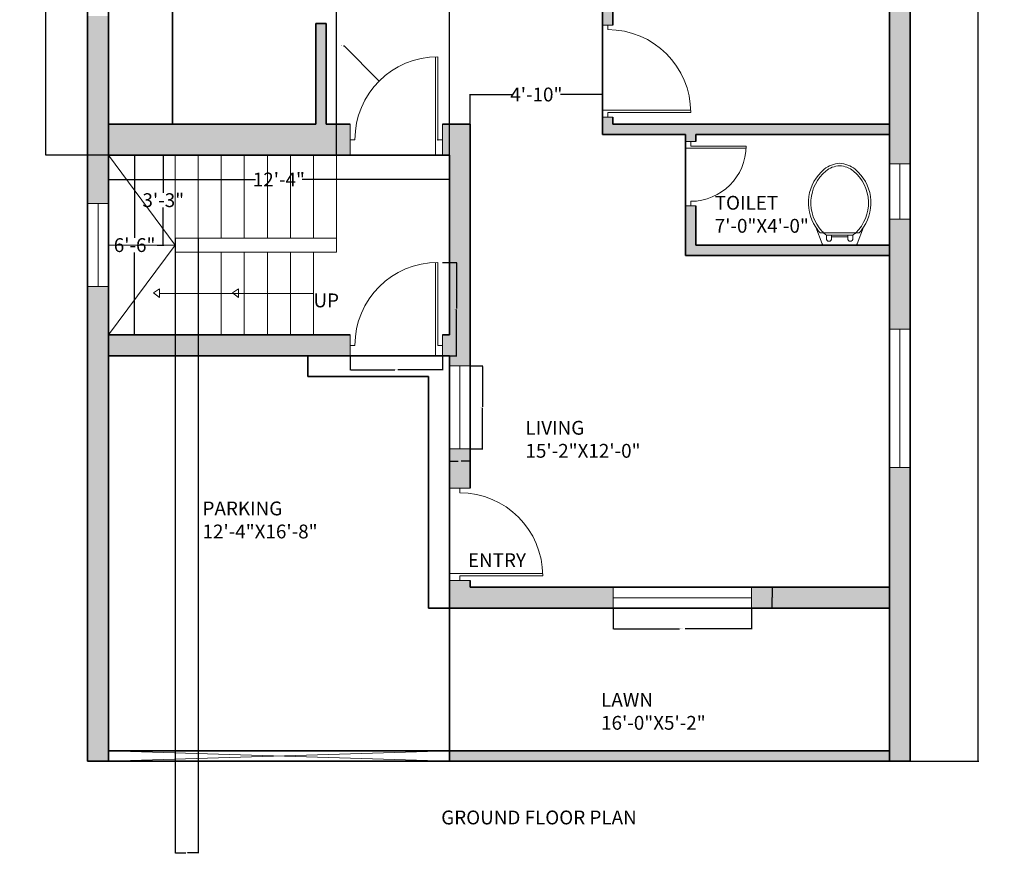
# Model space of a CAD drawing. Units: inches. Extents: x -15 to 423, y -713 to 71.
# Tile 1 of 24: x -4 to 423, y -713 to -351. Entities that reach past the tile are written whole.
import ezdxf

# ---------------------------------------------------------------- set-up
doc = ezdxf.new("R2010")
doc.units = ezdxf.units.IN
doc.header["$MEASUREMENT"] = 0
for name, color, linetype, lineweight in [('A-ANNO-DIMS', 2, 'Continuous', 18), ('A-ANNO-SYMB', 7, 'Continuous', 13), ('A-ANNO-TEXT', 7, 'Continuous', 18), ('A-AREA-IDEN', 7, 'Continuous', 18), ('A-DOOR', 3, 'Continuous', 18), ('A-FLOR-CASE', 7, 'Continuous', 25), ('A-FLOR-STRS', 7, 'Continuous', 18), ('A-GLAZ', 5, 'Continuous', 18), ('A-SITE-GATE', 1, 'Continuous', 18), ('A-WALL', 7, 'Continuous', 35), ('A-WALL-PATT', 8, 'Continuous', 13), ('WC-Detail_dwgmodels.com', 251, 'Continuous', 13), ('WC-Outline_dwgmodels.com', 250, 'Continuous', 18)]:
    doc.layers.add(name, color=color, linetype=linetype, lineweight=lineweight)
doc.styles.get("Standard").update_dxf_attribs({"font": 'arial.ttf'})
doc.dimstyles.get("Standard").update_dxf_attribs({"dimtxt": 0.18, "dimasz": 0.18, "dimexe": 0.18, "dimexo": 0.0625, "dimgap": 0.09, "dimtad": 0, "dimtih": 1, "dimtoh": 1, "dimdec": 0, "dimzin": 0, "dimdsep": 46, "dimlunit": 3, "dimtxsty": 'Standard', "dimcen": 0.09, "dimadec": 0, "dimazin": 0, "dimtfac": 1, "dimtdec": 0, "dimtofl": 0, "dimtmove": 0, "dimatfit": 3, "dimfxl": 1, "dimtolj": 1, "dimtzin": 0, "dimarcsym": 0})

# ---------------------------------------------------------------- blocks, each defined once
blk = doc.blocks.new('*D3')
at = {"layer": 'A-ANNO-DIMS', "color": 0, "lineweight": -2, "transparency": 16777216}
for p, q in [((34.08, -413.18), (34.08, -420.72)), ((182.08, -413.18), (182.08, -420.72)), ((34.26, -420.54), (97.97, -420.54)), ((181.9, -420.54), (118.19, -420.54))]:
    blk.add_line(p, q, dxfattribs=at)
at = {"layer": 'A-ANNO-DIMS', "color": 0, "transparency": 16777216}
for points in [[(34.26, -420.51), (34.26, -420.57), (34.08, -420.54)], [(181.9, -420.51), (181.9, -420.57), (182.08, -420.54)]]:
    blk.add_solid(points, dxfattribs=at)
at = {"layer": 'Defpoints', "color": 0, "transparency": 16777216}
for p in [(34.08, -413.12), (182.08, -413.12), (182.08, -420.54)]:
    blk.add_point(p, dxfattribs=at)
at = {"layer": 'A-ANNO-DIMS', "color": 0, "transparency": 16777216, "insert": (108.08, -420.54), "char_height": 6, "attachment_point": 5}
blk.add_mtext('\\A1;12\'-4"', dxfattribs=at)
blk = doc.blocks.new('*D4')
at = {"layer": 'A-ANNO-DIMS', "color": 0, "lineweight": -2, "transparency": 16777216}
for p, q in [((50.57, -410), (45.28, -410)), ((45.46, -410.18), (45.46, -445.85)), ((45.46, -487.82), (45.46, -452.15)), ((50.57, -488), (45.28, -488))]:
    blk.add_line(p, q, dxfattribs=at)
at = {"layer": 'A-ANNO-DIMS', "color": 0, "transparency": 16777216}
for points in [[(45.43, -410.18), (45.49, -410.18), (45.46, -410)], [(45.43, -487.82), (45.49, -487.82), (45.46, -488)]]:
    blk.add_solid(points, dxfattribs=at)
at = {"layer": 'Defpoints', "color": 0, "transparency": 16777216}
for p in [(50.63, -410), (45.46, -488), (50.63, -488)]:
    blk.add_point(p, dxfattribs=at)
at = {"layer": 'A-ANNO-DIMS', "color": 0, "transparency": 16777216, "insert": (45.46, -449), "char_height": 6, "attachment_point": 5}
blk.add_mtext('\\A1;6\'-6"', dxfattribs=at)
blk = doc.blocks.new('*D5')
at = {"layer": 'A-ANNO-DIMS', "color": 0, "lineweight": -2, "transparency": 16777216}
for p, q in [((55.24, -410), (58.09, -410)), ((57.91, -410.18), (57.91, -426.34)), ((57.91, -448.82), (57.91, -432.66)), ((55.24, -449), (58.09, -449))]:
    blk.add_line(p, q, dxfattribs=at)
at = {"layer": 'A-ANNO-DIMS', "color": 0, "transparency": 16777216}
for points in [[(57.88, -410.18), (57.94, -410.18), (57.91, -410)], [(57.88, -448.82), (57.94, -448.82), (57.91, -449)]]:
    blk.add_solid(points, dxfattribs=at)
at = {"layer": 'Defpoints', "color": 0, "transparency": 16777216}
for p in [(55.18, -410), (55.18, -449), (57.91, -449)]:
    blk.add_point(p, dxfattribs=at)
at = {"layer": 'A-ANNO-DIMS', "color": 0, "transparency": 16777216, "insert": (57.91, -429.5), "char_height": 6, "attachment_point": 5}
blk.add_mtext('\\A1;3\'-3"', dxfattribs=at)
blk = doc.blocks.new('*D6')
at = {"layer": 'A-ANNO-DIMS', "color": 0, "lineweight": -2, "transparency": 16777216}
for p, q in [((191.08, -396.44), (191.08, -383.46)), ((191.26, -383.64), (209.31, -383.64)), ((248.4, -383.64), (230.35, -383.64)), ((248.58, -393.44), (248.58, -383.46))]:
    blk.add_line(p, q, dxfattribs=at)
at = {"layer": 'A-ANNO-DIMS', "color": 0, "transparency": 16777216}
for points in [[(191.26, -383.61), (191.26, -383.67), (191.08, -383.64)], [(248.4, -383.61), (248.4, -383.67), (248.58, -383.64)]]:
    blk.add_solid(points, dxfattribs=at)
at = {"layer": 'Defpoints', "color": 0, "transparency": 16777216}
for p in [(248.58, -383.64), (191.08, -396.5), (248.58, -393.5)]:
    blk.add_point(p, dxfattribs=at)
at = {"layer": 'A-ANNO-DIMS', "color": 0, "transparency": 16777216, "insert": (219.83, -383.64), "char_height": 6, "attachment_point": 5}
blk.add_mtext('\\A1;4\'-10"', dxfattribs=at)
blk = doc.blocks.new('*D8')
at = {"layer": 'A-ANNO-DIMS', "color": 0, "lineweight": -2, "transparency": 16777216}
for p, q in [((25.02, 17.5), (6.72, 17.5)), ((6.9, 17.32), (6.9, -193.09)), ((6.9, -409.82), (6.9, -199.41)), ((34.02, -410), (6.72, -410))]:
    blk.add_line(p, q, dxfattribs=at)
at = {"layer": 'A-ANNO-DIMS', "color": 0, "transparency": 16777216}
for points in [[(6.87, 17.32), (6.93, 17.32), (6.9, 17.5)], [(6.87, -409.82), (6.93, -409.82), (6.9, -410)]]:
    blk.add_solid(points, dxfattribs=at)
at = {"layer": 'Defpoints', "color": 0, "transparency": 16777216}
for p in [(25.08, 17.5), (6.9, -410), (34.08, -410)]:
    blk.add_point(p, dxfattribs=at)
at = {"layer": 'A-ANNO-DIMS', "color": 0, "transparency": 16777216, "insert": (6.9, -196.25), "char_height": 6, "attachment_point": 5}
blk.add_mtext('\\A1;35\'-8"', dxfattribs=at)
blk = doc.blocks.new('*D9')
at = {"layer": 'A-ANNO-DIMS', "color": 0, "lineweight": -2, "transparency": 16777216}
for p, q in [((382.14, 17.5), (411.79, 17.5)), ((411.61, 17.32), (411.61, -324.61)), ((411.61, -672.82), (411.61, -330.89)), ((382.14, -673), (411.79, -673))]:
    blk.add_line(p, q, dxfattribs=at)
at = {"layer": 'A-ANNO-DIMS', "color": 0, "transparency": 16777216}
for points in [[(411.58, 17.32), (411.64, 17.32), (411.61, 17.5)], [(411.58, -672.82), (411.64, -672.82), (411.61, -673)]]:
    blk.add_solid(points, dxfattribs=at)
at = {"layer": 'Defpoints', "color": 0, "transparency": 16777216}
for p in [(382.08, 17.5), (382.08, -673), (411.61, -673)]:
    blk.add_point(p, dxfattribs=at)
at = {"layer": 'A-ANNO-DIMS', "color": 0, "transparency": 16777216, "insert": (411.61, -327.75), "char_height": 6, "attachment_point": 5}
blk.add_mtext('\\A1;57\'-7"', dxfattribs=at)
blk = doc.blocks.new('WINDOW-60IN')
for p, q in [((0, 9), (60, 9)), ((0, 0), (0, 9)), ((60, 9), (60, 0)), ((0, 4.5), (60, 4.5)), ((60, 0), (0, 0))]:
    blk.add_line(p, q)
blk = doc.blocks.new('WINDOW-24IN')
for p, q in [((9, 24), (0, 24)), ((0, 24), (0, 0)), ((4.5, 0), (4.5, 24)), ((9, 0), (9, 24)), ((0, 0), (9, 0))]:
    blk.add_line(p, q)
blk = doc.blocks.new('WINDOW-36IN')
for p, q in [((0, 36), (0, 0)), ((9, 36), (0, 36)), ((4.5, 36), (4.5, 0)), ((9, 0), (9, 36)), ((0, 0), (9, 0))]:
    blk.add_line(p, q)
blk = doc.blocks.new('DOOR-24IN-JAMB4_5')
for p, q in [((25, 0), (25, 26.25)), ((26, 2.25), (26, 26.25)), ((0, 2.25), (0, 4.5)), ((28, 4.5), (28, 0)), ((2, 2.25), (0, 2.25)), ((0, 2.25), (0, 0)), ((28, 2.25), (26, 2.25))]:
    blk.add_line(p, q)
blk.add_arc((26, 2.25), 24, 90, 180)
blk = doc.blocks.new('DOOR-36IN-JAMB4_5')
for p, q in [((2, 2.25), (2, 38.25)), ((3, 0), (3, 38.25)), ((0, 4.5), (0, 0)), ((40, 2.25), (40, 4.5)), ((0, 2.25), (2, 2.25)), ((38, 2.25), (40, 2.25)), ((40, 2.25), (40, 0))]:
    blk.add_line(p, q)
blk.add_arc((2, 2.25), 36, 0, 90)
blk = doc.blocks.new('DOOR-36IN-JAMB9')
for p, q in [((37, 0), (37, 40.5)), ((38, 4.5), (38, 40.5)), ((0, 4.5), (0, 9)), ((40, 9), (40, 0)), ((2, 4.5), (0, 4.5)), ((0, 4.5), (0, 0)), ((40, 4.5), (38, 4.5))]:
    blk.add_line(p, q)
blk.add_arc((38, 4.5), 36, 90, 180)
blk = doc.blocks.new('STAIR-DIRECTION-ARROW')
for p, q in [((2.56, 3.79), (0, 2.02)), ((0, 2.02), (2.56, 0)), ((2.56, 1.7), (2.56, 3.79)), ((2.56, 0), (2.56, 1.7))]:
    blk.add_line(p, q)
blk = doc.blocks.new('*D19')
at = {"layer": 'A-ANNO-DIMS', "color": 0, "lineweight": -2, "transparency": 16777216}
for p, q in [((253.2, -606.56), (253.2, -615.68)), ((313.2, -606.56), (313.2, -615.68)), ((253.38, -615.5), (281.97, -615.5)), ((313.02, -615.5), (284.43, -615.5))]:
    blk.add_line(p, q, dxfattribs=at)
at = {"layer": 'A-ANNO-DIMS', "color": 0, "transparency": 16777216}
for points in [[(253.38, -615.47), (253.38, -615.53), (253.2, -615.5)], [(313.02, -615.47), (313.02, -615.53), (313.2, -615.5)]]:
    blk.add_solid(points, dxfattribs=at)
at = {"layer": 'Defpoints', "color": 0, "transparency": 16777216}
for p in [(253.2, -606.5), (313.2, -606.5), (313.2, -615.5)]:
    blk.add_point(p, dxfattribs=at)
at = {"layer": 'A-ANNO-DIMS', "color": 0, "transparency": 16777216, "insert": (283.2, -615.5), "char_height": 0.18, "attachment_point": 5}
blk.add_mtext('\\A1;WINDOW 5\'-0" TYP.', dxfattribs=at)
blk = doc.blocks.new('*D20')
at = {"layer": 'A-ANNO-DIMS', "color": 0, "lineweight": -2, "transparency": 16777216}
for p, q in [((313.26, -597.5), (322.38, -597.5)), ((322.2, -597.68), (322.2, -601.82)), ((322.2, -606.32), (322.2, -602.18)), ((313.26, -606.5), (322.38, -606.5))]:
    blk.add_line(p, q, dxfattribs=at)
at = {"layer": 'A-ANNO-DIMS', "color": 0, "transparency": 16777216}
for points in [[(322.17, -597.68), (322.23, -597.68), (322.2, -597.5)], [(322.17, -606.32), (322.23, -606.32), (322.2, -606.5)]]:
    blk.add_solid(points, dxfattribs=at)
at = {"layer": 'Defpoints', "color": 0, "transparency": 16777216}
for p in [(313.2, -597.5), (322.2, -597.5), (313.2, -606.5)]:
    blk.add_point(p, dxfattribs=at)
at = {"layer": 'A-ANNO-DIMS', "color": 0, "transparency": 16777216, "insert": (322.2, -602), "char_height": 0.18, "attachment_point": 5}
blk.add_mtext('\\A1;0\'-9" TYP.', dxfattribs=at)
blk = doc.blocks.new('*D21')
at = {"layer": 'A-ANNO-DIMS', "color": 0, "lineweight": -2, "transparency": 16777216}
for p, q in [((191.14, -501.43), (196.66, -501.43)), ((196.48, -501.61), (196.48, -519.25)), ((196.48, -537.25), (196.48, -519.61)), ((191.14, -537.43), (196.66, -537.43))]:
    blk.add_line(p, q, dxfattribs=at)
at = {"layer": 'A-ANNO-DIMS', "color": 0, "transparency": 16777216}
for points in [[(196.45, -501.61), (196.51, -501.61), (196.48, -501.43)], [(196.45, -537.25), (196.51, -537.25), (196.48, -537.43)]]:
    blk.add_solid(points, dxfattribs=at)
at = {"layer": 'Defpoints', "color": 0, "transparency": 16777216}
for p in [(191.08, -501.43), (196.48, -501.43), (191.08, -537.43)]:
    blk.add_point(p, dxfattribs=at)
at = {"layer": 'A-ANNO-DIMS', "color": 0, "transparency": 16777216, "insert": (196.48, -519.43), "char_height": 0.18, "attachment_point": 5}
blk.add_mtext('\\A1;WINDOW 3\'-0" TYP.', dxfattribs=at)
blk = doc.blocks.new('*D22')
at = {"layer": 'A-ANNO-DIMS', "color": 0, "lineweight": -2, "transparency": 16777216}
for p, q in [((182.08, -537.49), (182.08, -543.01)), ((191.08, -537.49), (191.08, -543.01)), ((182.26, -542.83), (185.94, -542.83)), ((190.9, -542.83), (187.22, -542.83))]:
    blk.add_line(p, q, dxfattribs=at)
at = {"layer": 'A-ANNO-DIMS', "color": 0, "transparency": 16777216}
for points in [[(182.26, -542.8), (182.26, -542.86), (182.08, -542.83)], [(190.9, -542.8), (190.9, -542.86), (191.08, -542.83)]]:
    blk.add_solid(points, dxfattribs=at)
at = {"layer": 'Defpoints', "color": 0, "transparency": 16777216}
for p in [(182.08, -537.43), (191.08, -537.43), (191.08, -542.83)]:
    blk.add_point(p, dxfattribs=at)
at = {"layer": 'A-ANNO-DIMS', "color": 0, "transparency": 16777216, "insert": (186.58, -542.83), "char_height": 0.18, "attachment_point": 5}
blk.add_mtext('\\A1;0\'-9" TYP.', dxfattribs=at)
blk = doc.blocks.new('*D29')
at = {"layer": 'A-ANNO-DIMS', "color": 0, "lineweight": -2, "transparency": 16777216}
for p, q in [((179.14, -456.5), (185.34, -456.5)), ((185.16, -456.68), (185.16, -476.57)), ((185.16, -496.82), (185.16, -476.93)), ((179.14, -497), (185.34, -497))]:
    blk.add_line(p, q, dxfattribs=at)
at = {"layer": 'A-ANNO-DIMS', "color": 0, "transparency": 16777216}
for points in [[(185.13, -456.68), (185.19, -456.68), (185.16, -456.5)], [(185.13, -496.82), (185.19, -496.82), (185.16, -497)]]:
    blk.add_solid(points, dxfattribs=at)
at = {"layer": 'Defpoints', "color": 0, "transparency": 16777216}
for p in [(179.08, -456.5), (185.16, -456.5), (179.08, -497)]:
    blk.add_point(p, dxfattribs=at)
at = {"layer": 'A-ANNO-DIMS', "color": 0, "transparency": 16777216, "insert": (185.16, -476.75), "char_height": 0.18, "attachment_point": 5}
blk.add_mtext('\\A1;DOOR 3\'-4 1/2" TYP.', dxfattribs=at)
blk = doc.blocks.new('*D30')
at = {"layer": 'A-ANNO-DIMS', "color": 0, "lineweight": -2, "transparency": 16777216}
for p, q in [((139.08, -497.06), (139.08, -503.25)), ((179.08, -497.06), (179.08, -503.25)), ((139.26, -503.07), (158.44, -503.07)), ((178.9, -503.07), (159.72, -503.07))]:
    blk.add_line(p, q, dxfattribs=at)
at = {"layer": 'A-ANNO-DIMS', "color": 0, "transparency": 16777216}
for points in [[(139.26, -503.04), (139.26, -503.1), (139.08, -503.07)], [(178.9, -503.04), (178.9, -503.1), (179.08, -503.07)]]:
    blk.add_solid(points, dxfattribs=at)
at = {"layer": 'Defpoints', "color": 0, "transparency": 16777216}
for p in [(139.08, -497), (179.08, -497), (179.08, -503.07)]:
    blk.add_point(p, dxfattribs=at)
at = {"layer": 'A-ANNO-DIMS', "color": 0, "transparency": 16777216, "insert": (159.08, -503.07), "char_height": 0.18, "attachment_point": 5}
blk.add_mtext('\\A1;3\'-4" TYP.', dxfattribs=at)
blk = doc.blocks.new('*D37')
at = {"layer": 'A-ANNO-DIMS', "color": 0, "lineweight": -2, "transparency": 16777216}
for p, q in [((34.08, -396.44), (34.08, 57.43)), ((34.26, 57.25), (47.65, 57.25)), ((61.7, 57.25), (48.31, 57.25)), ((61.88, -396.44), (61.88, 57.43))]:
    blk.add_line(p, q, dxfattribs=at)
at = {"layer": 'A-ANNO-DIMS', "color": 0, "transparency": 16777216}
for points in [[(34.26, 57.28), (34.26, 57.22), (34.08, 57.25)], [(61.7, 57.28), (61.7, 57.22), (61.88, 57.25)]]:
    blk.add_solid(points, dxfattribs=at)
at = {"layer": 'Defpoints', "color": 0, "transparency": 16777216}
for p in [(61.88, 57.25), (34.08, -396.5), (61.88, -396.5)]:
    blk.add_point(p, dxfattribs=at)
at = {"layer": 'A-ANNO-DIMS', "color": 0, "transparency": 16777216, "insert": (47.98, 57.25), "char_height": 0.18, "attachment_point": 5}
blk.add_mtext('\\A1;2\'-4"', dxfattribs=at)
blk = doc.blocks.new('*D41')
at = {"layer": 'A-ANNO-DIMS', "color": 0, "lineweight": -2, "transparency": 16777216}
for p, q in [((63.08, -446.06), (63.08, -712.93)), ((73.08, -446.06), (73.08, -712.93)), ((63.26, -712.75), (67.68, -712.75)), ((72.9, -712.75), (68.48, -712.75))]:
    blk.add_line(p, q, dxfattribs=at)
at = {"layer": 'A-ANNO-DIMS', "color": 0, "transparency": 16777216}
for points in [[(63.26, -712.72), (63.26, -712.78), (63.08, -712.75)], [(72.9, -712.72), (72.9, -712.78), (73.08, -712.75)]]:
    blk.add_solid(points, dxfattribs=at)
at = {"layer": 'Defpoints', "color": 0, "transparency": 16777216}
for p in [(63.08, -446), (73.08, -446), (73.08, -712.75)]:
    blk.add_point(p, dxfattribs=at)
at = {"layer": 'A-ANNO-DIMS', "color": 0, "transparency": 16777216, "insert": (68.08, -712.75), "char_height": 0.18, "attachment_point": 5}
blk.add_mtext('\\A1;0\'-10"', dxfattribs=at)
blk = doc.blocks.new('*D42')
at = {"layer": 'A-ANNO-DIMS', "color": 0, "lineweight": -2, "transparency": 16777216}
for p, q in [((133.08, -409.94), (133.08, 57.43)), ((133.26, 57.25), (157.25, 57.25)), ((181.9, 57.25), (157.91, 57.25)), ((182.08, -409.94), (182.08, 57.43))]:
    blk.add_line(p, q, dxfattribs=at)
at = {"layer": 'A-ANNO-DIMS', "color": 0, "transparency": 16777216}
for points in [[(133.26, 57.28), (133.26, 57.22), (133.08, 57.25)], [(181.9, 57.28), (181.9, 57.22), (182.08, 57.25)]]:
    blk.add_solid(points, dxfattribs=at)
at = {"layer": 'Defpoints', "color": 0, "transparency": 16777216}
for p in [(182.08, 57.25), (133.08, -410), (182.08, -410)]:
    blk.add_point(p, dxfattribs=at)
at = {"layer": 'A-ANNO-DIMS', "color": 0, "transparency": 16777216, "insert": (157.58, 57.25), "char_height": 0.18, "attachment_point": 5}
blk.add_mtext('\\A1;4\'-1"', dxfattribs=at)
blk = doc.blocks.new('*D43')
at = {"layer": 'A-ANNO-DIMS', "color": 0, "lineweight": -2, "transparency": 16777216}
for p, q in [((136.17, -362.52), (136.35, -362.52)), ((136.35, -362.52), (151.5, -377.67)), ((176.99, -403.25), (177.17, -403.25)), ((177.08, -403.34), (177.08, -403.16))]:
    blk.add_line(p, q, dxfattribs=at)
at = {"layer": 'A-ANNO-DIMS', "color": 0, "transparency": 16777216}
blk.add_solid([(151.52, -377.65), (151.48, -377.69), (151.62, -377.79)], dxfattribs=at)
at = {"layer": 'Defpoints', "color": 0, "transparency": 16777216}
for p in [(151.62, -377.79), (177.08, -403.25)]:
    blk.add_point(p, dxfattribs=at)
at = {"layer": 'A-ANNO-DIMS', "color": 0, "transparency": 16777216, "insert": (135.56, -362.52), "char_height": 0.18, "attachment_point": 5}
blk.add_mtext('\\A1;3X R3\'-0"', dxfattribs=at)

msp = doc.modelspace()

# ---------------------------------------------------------------- hatches: boundary and pattern name
at = {"layer": 'A-WALL-PATT'}
h = msp.add_hatch(color=256, dxfattribs=at)
h.dxf.hatch_style = 1
h.paths.add_polyline_path([(34.08, -349.58), (25.08, -349.58), (25.08, -431), (34.08, -431)])
h.paths.add_polyline_path([(34.08, -467), (25.08, -467), (25.08, -673), (34.08, -673)])
h.paths.add_polyline_path([(373.08, -668.5), (182.08, -668.5), (182.08, -673), (373.08, -673)])
h.paths.add_polyline_path([(253.2, -597.5), (191.08, -597.5), (191.08, -594.5), (182.08, -594.5), (182.08, -606.5), (253.2, -606.5)])
h.paths.add_polyline_path([(373.08, -597.5), (313.2, -597.5), (313.2, -606.5), (373.08, -606.5)])
h.paths.add_polyline_path([(382.08, -545.55), (373.08, -545.55), (373.08, -673), (382.08, -673)])
h.paths.add_polyline_path([(139.08, -488), (34.08, -488), (34.08, -497), (139.08, -497), (139.08, -492.5)])
h.paths.add_polyline_path([(139.08, -396.5), (128.58, -396.5), (128.58, -352.79), (124.08, -352.79), (124.08, -396.5), (34.08, -396.5), (34.08, -410), (139.08, -410), (139.08, -403.25)])
h.paths.add_polyline_path([(191.08, -396.5), (179.08, -396.5), (179.08, -410), (182.08, -410), (182.08, -488), (179.08, -488), (179.08, -497), (182.08, -497), (182.08, -501.43), (191.08, -501.43)])
h.paths.add_polyline_path([(373.08, -396.5), (253.08, -396.5), (253.08, -393.5), (248.58, -393.5), (248.58, -401), (284.58, -401), (284.58, -404), (289.08, -404), (289.08, -401), (373.08, -401)])
h.paths.add_polyline_path([(373.08, -449), (289.08, -449), (289.08, -432), (286.83, -432), (284.58, -432), (284.58, -453.5), (373.08, -453.5)])
h.paths.add_polyline_path([(382.08, -344.27), (373.08, -344.27), (373.08, -413.68), (382.08, -413.68)])
h.paths.add_polyline_path([(382.08, -437.68), (373.08, -437.68), (373.08, -485.55), (382.08, -485.55)])
h.paths.add_polyline_path([(34.08, -188.26), (25.08, -188.26), (25.08, -289.58), (34.08, -289.58)])
h.paths.add_polyline_path([(164.08, -236), (34.08, -236), (34.08, -240.5), (124.08, -240.5), (124.08, -293.12), (128.58, -293.12), (128.58, -240.5), (164.08, -240.5), (164.08, -238.25)])
h.paths.add_polyline_path([(373.08, -236), (242.58, -236), (242.58, -238.25), (242.58, -240.5), (248.58, -240.5), (248.58, -353.5), (250.83, -353.5), (253.08, -353.5), (253.08, -240.5), (373.08, -240.5)])
h.paths.add_polyline_path([(382.08, -190.86), (373.08, -190.86), (373.08, -284.27), (382.08, -284.27)])
h.paths.add_polyline_path([(211.58, -80), (253.58, -80), (253.58, -77.75), (253.58, -75.5), (153.58, -75.5), (153.58, -77.75), (153.58, -80), (207.08, -80), (207.08, -236), (204.08, -236), (204.08, -240.5), (214.58, -240.5), (214.58, -236), (211.58, -236)])
h.paths.add_polyline_path([(34.08, 8.5), (70.36, 8.5), (70.36, 17.5), (25.08, 17.5), (25.08, -128.26), (34.08, -128.26)])
h.paths.add_polyline_path([(110.58, 17.5), (94.36, 17.5), (94.36, 8.5), (110.58, 8.5)])
h.paths.add_polyline_path([(296.58, 17.5), (110.58, 17.5), (110.58, 13), (296.58, 13)])
h.paths.add_polyline_path([(110.58, 8.5), (106.08, 8.5), (106.08, -75.5), (103.08, -75.5), (103.08, -80), (113.58, -80), (113.58, -77.75), (113.58, -75.5), (110.58, -75.5)])
h.paths.add_polyline_path([(75.08, -75.5), (34.08, -75.5), (34.08, -80), (75.08, -80), (75.08, -77.75)])
h.paths.add_polyline_path([(343.09, 17.5), (296.58, 17.5), (296.58, 13), (296.58, 8.5), (343.09, 8.5)])
h.paths.add_polyline_path([(304.08, -75.5), (301.08, -75.5), (301.08, 8.5), (296.58, 8.5), (296.58, -75.5), (293.58, -75.5), (293.58, -80), (304.08, -80)])
h.paths.add_polyline_path([(382.08, 17.5), (367.09, 17.5), (367.09, 8.5), (373.08, 8.5), (373.08, -130.86), (382.08, -130.86)])
h.paths.add_polyline_path([(373.08, -75.5), (332.08, -75.5), (332.08, -77.75), (332.08, -80), (373.08, -80)])
h = msp.add_hatch(color=256, dxfattribs=at)
h.dxf.hatch_style = 1
h.paths.add_polyline_path([(191.08, -537.43), (182.08, -537.43), (182.08, -554.5), (186.58, -554.5), (191.08, -554.5)])

# ---------------------------------------------------------------- linework, layer by layer
at = {"layer": 'A-ANNO-SYMB'}
msp.add_line((123.08, -470), (56.22, -470), dxfattribs=at)
at = {"layer": 'A-DOOR'}
for p, q in [((176.08, -410), (176.08, -367.25)), ((177.08, -403.25), (177.08, -367.25)), ((139.08, -403.25), (139.08, -396.5)), ((179.08, -410), (179.08, -396.5)), ((141.08, -403.25), (139.08, -403.25)), ((139.08, -403.25), (139.08, -410)), ((179.08, -403.25), (177.08, -403.25))]:
    msp.add_line(p, q, dxfattribs=at)
msp.add_arc((177.08, -403.25), 36, 90, 180, dxfattribs=at)
at = {"layer": 'A-FLOR-CASE'}
msp.add_line((61.88, -275.98), (61.88, -396.5), dxfattribs=at)
at = {"layer": 'A-FLOR-STRS'}
for p, q in [((63.08, -449), (34.08, -410)), ((63.08, -410), (63.08, -488)), ((73.08, -410), (73.08, -446)), ((83.08, -410), (83.08, -446)), ((93.08, -410), (93.08, -446)), ((103.08, -410), (103.08, -446)), ((113.08, -410), (113.08, -446)), ((123.08, -410), (123.08, -446)), ((133.08, -410), (133.08, -452)), ((63.08, -446), (133.08, -446)), ((63.08, -449), (34.08, -449)), ((63.08, -449), (34.08, -488)), ((63.08, -452), (133.08, -452)), ((73.08, -452), (73.08, -488)), ((83.08, -452), (83.08, -488)), ((93.08, -452), (93.08, -488)), ((103.08, -452), (103.08, -488)), ((113.08, -452), (113.08, -488)), ((123.08, -452), (123.08, -488))]:
    msp.add_line(p, q, dxfattribs=at)
at = {"layer": 'A-SITE-GATE'}
for p, q in [((34.08, -668.5), (182.08, -673)), ((182.08, -668.5), (34.08, -673))]:
    msp.add_line(p, q, dxfattribs=at)
at = {"layer": 'A-WALL'}
for p, q in [((25.08, 17.5), (25.08, -673)), ((382.08, 17.5), (382.08, -673)), ((34.08, 8.5), (34.08, -673)), ((373.08, 8.5), (373.08, -673)), ((248.58, -240.5), (248.58, -401)), ((253.08, -240.5), (253.08, -353.5)), ((124.08, -352.79), (128.58, -352.79)), ((124.08, -352.79), (124.08, -396.5)), ((128.58, -352.79), (128.58, -396.5)), ((34.08, -396.5), (124.08, -396.5)), ((128.58, -396.5), (139.08, -396.5)), ((179.08, -396.5), (191.08, -396.5)), ((191.08, -396.5), (191.08, -554.5)), ((253.08, -393.5), (253.08, -396.5)), ((253.08, -396.5), (373.08, -396.5)), ((248.58, -401), (284.58, -401)), ((284.58, -401), (284.58, -453.5)), ((289.08, -401), (373.08, -401)), ((289.08, -401), (289.08, -404)), ((34.08, -410), (182.08, -410)), ((182.08, -410), (182.08, -488)), ((289.08, -432), (289.08, -449)), ((289.08, -449), (373.08, -449)), ((284.58, -453.5), (373.08, -453.5)), ((34.08, -488), (139.08, -488)), ((179.08, -488), (182.08, -488)), ((34.08, -497), (182.08, -497)), ((120.64, -497), (120.64, -506)), ((182.08, -497), (182.08, -668.5)), ((120.64, -506), (173.08, -506)), ((173.08, -506), (173.08, -606.5)), ((191.08, -594.5), (191.08, -597.5)), ((191.08, -597.5), (373.08, -597.5)), ((173.08, -606.5), (182.08, -606.5)), ((182.08, -606.5), (373.08, -606.5)), ((34.08, -668.5), (373.08, -668.5)), ((182.08, -668.5), (182.08, -673)), ((25.08, -673), (382.08, -673))]:
    msp.add_line(p, q, dxfattribs=at)
at = {"layer": 'WC-Detail_dwgmodels.com'}
for p, q in [((342.98, -443.63), (344.47, -443.63)), ((358.44, -443.63), (359.93, -443.63))]:
    msp.add_line(p, q, dxfattribs=at)
for points in [[(342.98, -443.63, -0.040937), (341.06, -441.19, -0.163732)], [(345.7, -444.7, -0.022712), (344.47, -443.63, -0.162618)], [(357.21, -444.7, 0.022712), (358.44, -443.63, 0.162618)], [(359.93, -443.63, 0.040937), (361.85, -441.19, 0.163732)], [(351.45, -444.7), (345.7, -444.7, -0.022712)], [(345.7, -444.7), (345.7, -446.19, 1), (347.96, -446.19), (347.96, -445.41)], [(351.45, -444.7), (357.21, -444.7, 0.476108)], [(357.21, -444.7), (357.21, -446.19, -1), (354.95, -446.19), (354.95, -445.41)]]:
    msp.add_lwpolyline(points, format="xyb", dxfattribs=at)
for points in [[(347.96, -445.41), (347.96, -444.7)], [(354.95, -445.41), (347.96, -445.41)], [(354.95, -445.41), (354.95, -444.7)]]:
    msp.add_lwpolyline(points, dxfattribs=at)
at = {"layer": 'WC-Outline_dwgmodels.com'}
for p in [(344.47, -443.63), (358.44, -443.63)]:
    msp.add_line(p, (351.45, -443.63), dxfattribs=at)
for points in [[(341.06, -441.19, -0.383919), (344.78, -416.07, -0.163732), (351.45, -413.51, -0.359733)], [(361.85, -441.19, 0.383919), (358.13, -416.07, 0.163732), (351.45, -413.51, 0.359733)], [(343.76, -442.9, -0.431639), (345.46, -416.88, -0.162618), (351.45, -414.57, -0.470877)], [(358.44, -443.63, 0.448546), (357.45, -416.88, 0.162618), (351.45, -414.57, 0.470877)], [(351.45, -449), (344.68, -449, -0.31031), (343.85, -448.43), (341.06, -441.19, -0.209071)], [(344.47, -443.63, -0.014165), (343.76, -442.9, -0.162618)], [(351.45, -449), (358.23, -449, 0.31031), (359.06, -448.43), (361.85, -441.19, 0.209071)]]:
    msp.add_lwpolyline(points, format="xyb", dxfattribs=at)

# ---------------------------------------------------------------- block references
at = {"layer": 'A-ANNO-SYMB'}
for p in [(53.66, -471.7), (88.01, -471.7)]:
    msp.add_blockref('STAIR-DIRECTION-ARROW', p, dxfattribs=at)
at = {"layer": 'A-DOOR', "extrusion": (0, 0, -1), "zscale": -1, "rotation": 90.00000000000003}
for name, p in [('DOOR-36IN-JAMB4_5', (-248.58, -393.5)), ('DOOR-24IN-JAMB4_5', (-284.58, -432))]:
    msp.add_blockref(name, p, dxfattribs=at)
at = {"layer": 'A-DOOR'}
msp.add_blockref('DOOR-36IN-JAMB9', (139.08, -497), dxfattribs=at)
at = {"layer": 'A-DOOR', "rotation": 270}
msp.add_blockref('DOOR-36IN-JAMB9', (182.08, -554.5), dxfattribs=at)
at = {"layer": 'A-GLAZ'}
for name, p in [('WINDOW-24IN', (373.08, -437.68)), ('WINDOW-36IN', (25.08, -467)), ('WINDOW-36IN', (182.08, -537.43)), ('WINDOW-60IN', (253.2, -606.5))]:
    msp.add_blockref(name, p, dxfattribs=at)
at = {"layer": 'A-GLAZ', "rotation": 90.00000000000011}
msp.add_blockref('WINDOW-60IN', (382.08, -545.55), dxfattribs=at)

# ---------------------------------------------------------------- texts
at = {"layer": 'A-ANNO-TEXT', "char_height": 6, "attachment_point": 1}
for s, insert in [('UP', (123.08, -470)), ('GROUND FLOOR PLAN', (178.53, -694.38))]:
    msp.add_mtext(s, dxfattribs=dict(at, insert=insert))
at = {"layer": 'A-AREA-IDEN', "char_height": 6, "attachment_point": 1}
for s, insert in [('TOILET\\P7\'-0"X4\'-0"', (297.24, -427.63)), ('LIVING\\P15\'-2"X12\'-0"', (215.1, -525.27)), ('PARKING\\P12\'-4"X16\'-8"', (74.94, -560.28)), ('ENTRY', (190.13, -582.75)), ('LAWN\\P16\'-0"X5\'-2"', (247.92, -643.31))]:
    msp.add_mtext(s, dxfattribs=dict(at, insert=insert))

# ---------------------------------------------------------------- dimensions: what is measured, and where the dimension line sits
at = {"layer": 'A-ANNO-DIMS'}
for base, p1, p2, override, picture, middle in [((61.88, 57.25), (34.08, -396.5), (61.88, -396.5), {"dimdec": 1, "dimlfac": 1, "dimrnd": 0, "dimzin": 1, "dimdsep": 46, "dimlunit": 4, "dimfrac": 2}, '*D37', (47.98, 57.25)), ((182.08, 57.25), (133.08, -410), (182.08, -410), {"dimdec": 1, "dimlfac": 1, "dimrnd": 0, "dimzin": 1, "dimdsep": 46, "dimlunit": 4, "dimfrac": 2}, '*D42', (157.58, 57.25)), ((248.58055573, -383.64367342), (191.08055573, -396.49989936), (248.58055573, -393.49989936), {"dimtxt": 6, "dimclrd": 0, "dimclre": 0, "dimclrt": 0}, '*D6', (219.83055573, -383.64367342)), ((182.08, -420.54), (34.08, -413.12), (182.08, -413.12), {"dimtxt": 6, "dimclrd": 0, "dimclre": 0, "dimclrt": 0}, '*D3', (108.08, -420.54)), ((73.08, -712.75), (63.08, -446), (73.08, -446), {"dimdec": 1, "dimlfac": 1, "dimrnd": 0, "dimzin": 1, "dimdsep": 46, "dimlunit": 4, "dimfrac": 2}, '*D41', (68.08, -712.75))]:
    dim = msp.add_linear_dim(base=base, p1=p1, p2=p2, dimstyle='Standard', override=override, dxfattribs=at)
    dim.commit()
    dim.dimension.update_dxf_attribs({"geometry": picture, "text_midpoint": middle})
for base, p1, p2, picture, middle in [((6.9041327, -409.99989936), (25.08055573, 17.50010064), (34.08055573, -409.99989936), '*D8', (6.9041327, -196.24989936)), ((411.6050599, -672.99989936), (382.08055573, 17.50010064), (382.08055573, -672.99989936), '*D9', (411.6050599, -327.74989936)), ((45.46, -488), (50.63, -410), (50.63, -488), '*D4', (45.46, -449)), ((57.91, -449), (55.18, -410), (55.18, -449), '*D5', (57.91, -429.5))]:
    dim = msp.add_linear_dim(base=base, p1=p1, p2=p2, angle=90, dimstyle='Standard', override={"dimtxt": 6, "dimclrd": 0, "dimclre": 0, "dimclrt": 0}, dxfattribs=at)
    dim.commit()
    dim.dimension.update_dxf_attribs({"geometry": picture, "text_midpoint": middle})
dim = msp.add_radius_dim(center=(177.08, -403.25), mpoint=(151.62, -377.79), text='3X <>', dimstyle='Standard', override={"dimdec": 1, "dimlfac": 1, "dimrnd": 0, "dimzin": 1, "dimdsep": 46, "dimlunit": 4, "dimfrac": 2}, dxfattribs=at)
dim.commit()
dim.dimension.update_dxf_attribs({"geometry": '*D43', "text_midpoint": (135.56, -362.52), "dimtype": 164})
for base, p1, p2, text, picture, middle in [((185.16, -456.5), (179.08, -497), (179.08, -456.5), 'DOOR <> TYP.', '*D29', (185.16, -476.75)), ((196.48, -501.43), (191.08, -537.43), (191.08, -501.43), 'WINDOW <> TYP.', '*D21', (196.48, -519.43)), ((322.2, -597.5), (313.2, -606.5), (313.2, -597.5), '<> TYP.', '*D20', (322.2, -602))]:
    dim = msp.add_linear_dim(base=base, p1=p1, p2=p2, angle=90, text=text, dimstyle='Standard', override={"dimdec": 1, "dimlfac": 1, "dimrnd": 0, "dimzin": 1, "dimdsep": 46, "dimlunit": 4, "dimfrac": 2}, dxfattribs=at)
    dim.commit()
    dim.dimension.update_dxf_attribs({"geometry": picture, "text_midpoint": middle})
for base, p1, p2, text, picture, middle in [((179.08, -503.07), (139.08, -497), (179.08, -497), '<> TYP.', '*D30', (159.08, -503.07)), ((191.08, -542.83), (182.08, -537.43), (191.08, -537.43), '<> TYP.', '*D22', (186.58, -542.83)), ((313.2, -615.5), (253.2, -606.5), (313.2, -606.5), 'WINDOW <> TYP.', '*D19', (283.2, -615.5))]:
    dim = msp.add_linear_dim(base=base, p1=p1, p2=p2, text=text, dimstyle='Standard', override={"dimdec": 1, "dimlfac": 1, "dimrnd": 0, "dimzin": 1, "dimdsep": 46, "dimlunit": 4, "dimfrac": 2}, dxfattribs=at)
    dim.commit()
    dim.dimension.update_dxf_attribs({"geometry": picture, "text_midpoint": middle})

doc.saveas('drawing.dxf')
